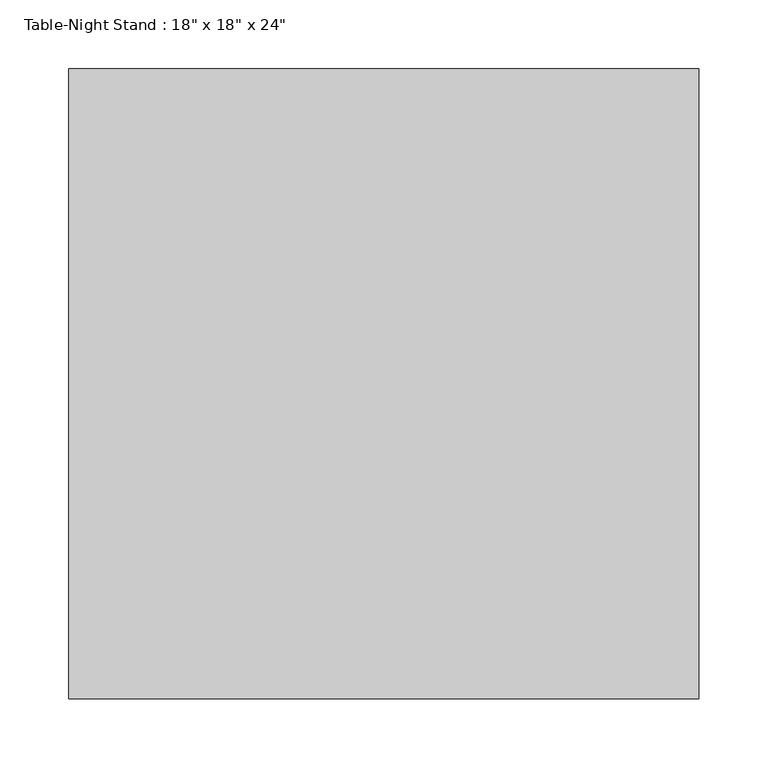
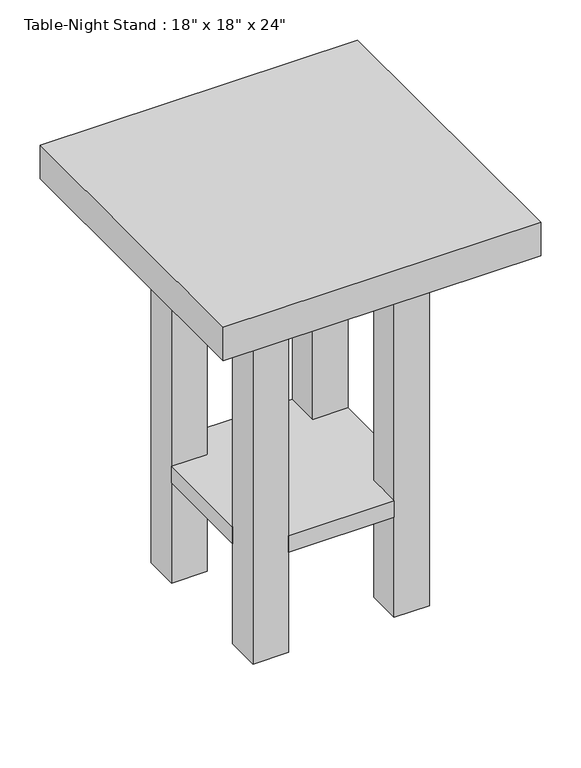
"""IFC4 building model written with IfcOpenShell, lengths in millimetres: furniture geometry."""

from ifc_helpers import new_model, si_unit, frame, origin, origin_with_axes, place, context, project, spatial, polyline, outline, extrude, source, transform, mapped, element, save


def furniture_097b63cf(model_context):
    return source(origin(), model_context, "Body", "SweptSolid", [
        extrude(outline(polyline([(156.1336303, 355.6), (308.5336303, 355.6), (308.5336303, 304.8), (359.3336303, 304.8), (359.3336303, 152.4), (308.5336303, 152.4), (308.5336303, 101.6), (156.1336303, 101.6), (156.1336303, 152.4), (105.3336303, 152.4), (105.3336303, 304.8), (156.1336303, 304.8), (156.1336303, 355.6)])), frame((0.0, 0.0, 152.4), z_axis=(0.0, 0.0, 1.0), x_axis=(1.0, 0.0, 0.0)), (0.0, 0.0, 1.0), 25.4),
        extrude(outline(polyline([(156.1336303, 355.6), (156.1336303, 304.8), (105.3336303, 304.8), (105.3336303, 355.6), (156.1336303, 355.6)])), origin_with_axes(), (0.0, 0.0, 1.0), 558.8),
        extrude(outline(polyline([(156.1336303, 152.4), (156.1336303, 101.6), (105.3336303, 101.6), (105.3336303, 152.4), (156.1336303, 152.4)])), origin_with_axes(), (0.0, 0.0, 1.0), 558.8),
        extrude(outline(polyline([(359.3336303, 355.6), (359.3336303, 304.8), (308.5336303, 304.8), (308.5336303, 355.6), (359.3336303, 355.6)])), origin_with_axes(), (0.0, 0.0, 1.0), 558.8),
        extrude(outline(polyline([(359.3336303, 152.4), (359.3336303, 101.6), (308.5336303, 101.6), (308.5336303, 152.4), (359.3336303, 152.4)])), origin_with_axes(), (0.0, 0.0, 1.0), 558.8),
        extrude(outline(polyline([(460.9336303, 0.0), (3.7336303, 0.0), (3.7336303, 457.2), (460.9336303, 457.2), (460.9336303, 0.0)])), frame((0.0, 0.0, 558.8), z_axis=(0.0, 0.0, 1.0), x_axis=(1.0, 0.0, 0.0)), (0.0, 0.0, 1.0), 50.8),
    ])


if __name__ == "__main__":
    model = new_model("IFC4")
    model_context = context("Model", 3, world=origin())
    ifc_project = project(units=[si_unit("LENGTHUNIT", "METRE", prefix="MILLI")], contexts=[model_context])
    site = spatial("IfcSite", under=ifc_project)
    building = spatial("IfcBuilding", under=site)
    placement = place(None, origin())
    furniture_shape = furniture_097b63cf(model_context)
    element("IfcFurniture", 1, ObjectType="Table-Night Stand : 18\" x 18\" x 24\"", at=placement, inside=building, context=model_context, shape_type="MappedRepresentation", body=[
        mapped(furniture_shape, transform((0.0, 0.0, 0.0), x_axis=(1.0, 0.0, 0.0), y_axis=(0.0, 1.0, 0.0), z_axis=(0.0, 0.0, 1.0))),
    ])
    save(model, "model.ifc")

# Revit data of these elements
# Type "Table-Night Stand : 18\" x 18\" x 24\""
#   Assembly Code = "E2020200"
#   Depth = 1' - 6"
#   Height = 2' - 0"
#   Width = 1' - 6"
#   Base Material = Birch
#   Top Material = Laminate, Ivory, Matte
#   Default Elevation = 0
# Element 1 (IfcFurniture, "Table-Night Stand : 18\" x 18\" x 24\"")
#   Materials on its faces: "Birch", "Laminate, Ivory, Matte"
# Materials
#   "Birch": class "Wood", colour RGB 224 178 126, transparency 0, Description = "Betula Alleghaniensis", Cost = 0
#   "Laminate, Ivory, Matte": class "Plastic", colour RGB 247 247 239, transparency 0, Description = "Plastic Laminate - Ivory, Matte", Cost = 0
